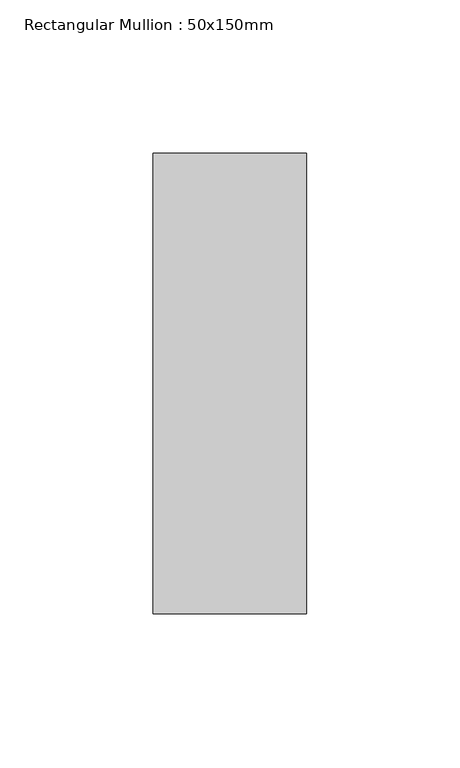
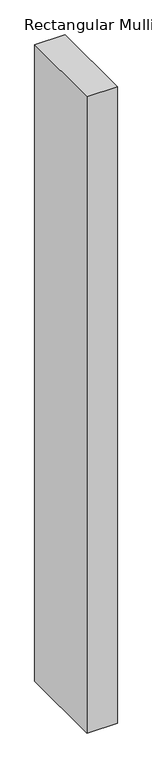
"""IFC4 building model written with IfcOpenShell, lengths in millimetres: member geometry, Rectangular Mullion : 50x150mm."""

from ifc_helpers import new_model, si_unit, frame, origin, place, context, project, spatial, polyline, outline, extrude, source, transform, mapped, element, save


def rectangular_mullion_50x150mm_024f1578(model_context):
    return source(origin(), model_context, "Body", "SweptSolid", [
        extrude(outline(polyline([(0.0, 75.0), (0.0, -75.0), (-50.0, -75.0), (-50.0, 75.0), (0.0, 75.0)])), frame((0.0, 0.0, -1112.218874), z_axis=(0.0, 0.0, 1.0), x_axis=(1.0, 0.0, 0.0)), (0.0, 0.0, 1.0), 1112.218874),
    ])


if __name__ == "__main__":
    model = new_model("IFC4")
    model_context = context("Model", 3, world=origin())
    ifc_project = project(units=[si_unit("LENGTHUNIT", "METRE", prefix="MILLI")], contexts=[model_context])
    site = spatial("IfcSite", under=ifc_project)
    building = spatial("IfcBuilding", under=site)
    placement = place(None, origin())
    rectangular_mullion_50x150mm_shape = rectangular_mullion_50x150mm_024f1578(model_context)
    element("IfcMember", 1, ObjectType="Rectangular Mullion : 50x150mm", at=placement, inside=building, context=model_context, shape_type="MappedRepresentation", body=[
        mapped(rectangular_mullion_50x150mm_shape, transform((0.0, 0.0, 0.0), x_axis=(1.0, 0.0, 0.0), y_axis=(0.0, 1.0, 0.0), z_axis=(0.0, 0.0, 1.0))),
    ])
    save(model, "model.ifc")

# Revit data of these elements
# Type "Rectangular Mullion : 50x150mm"
#   Keynote = "H11"
#   built-in parameter 1007304 = 0.492126 (stored number, unit not read)
#   built-in parameter 1007301 = 0.082021 (stored number, unit not read)
#   built-in parameter 1007300 = 0.082021 (stored number, unit not read)
# Element 1 (IfcMember, "Rectangular Mullion : 50x150mm")
#   Materials on its faces: "Aluminium"
# Materials
#   "Aluminium": class "Metal", colour RGB 247 247 247, transparency 0, Description = "Aluminium 6061", Cost = 0
